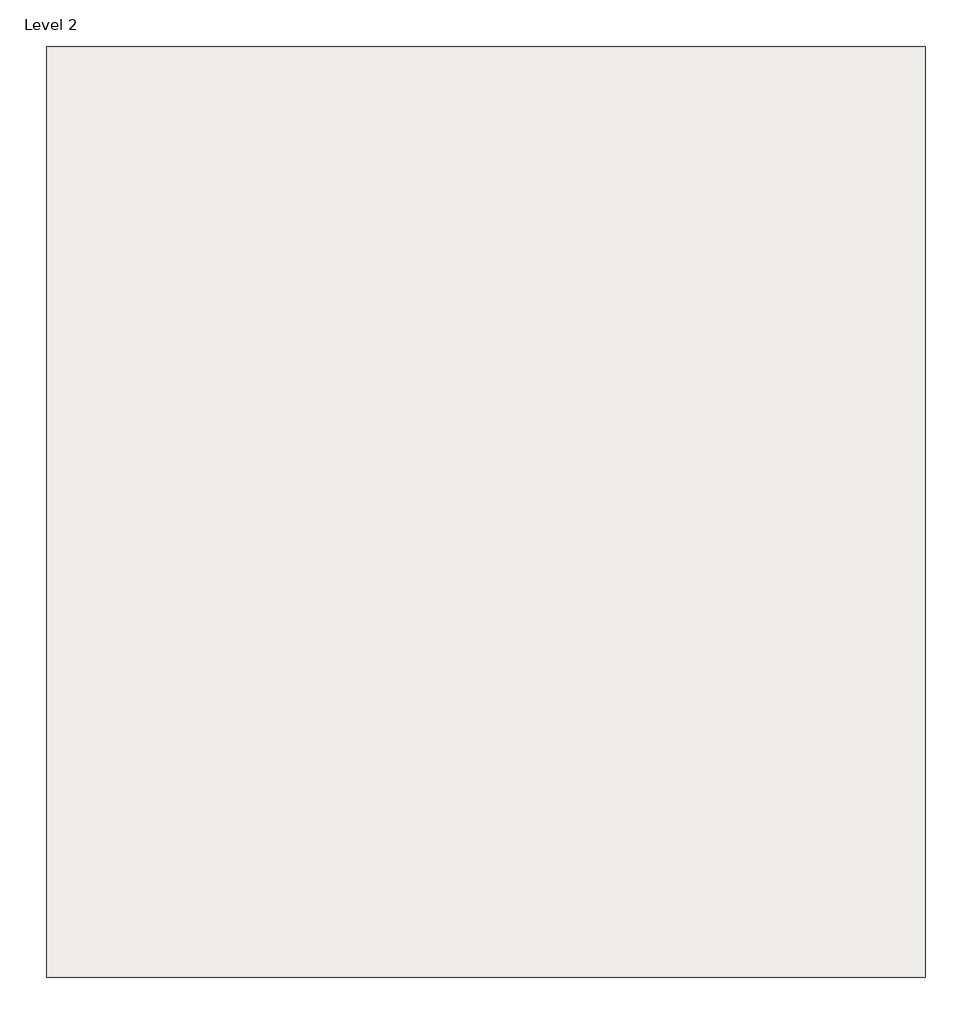
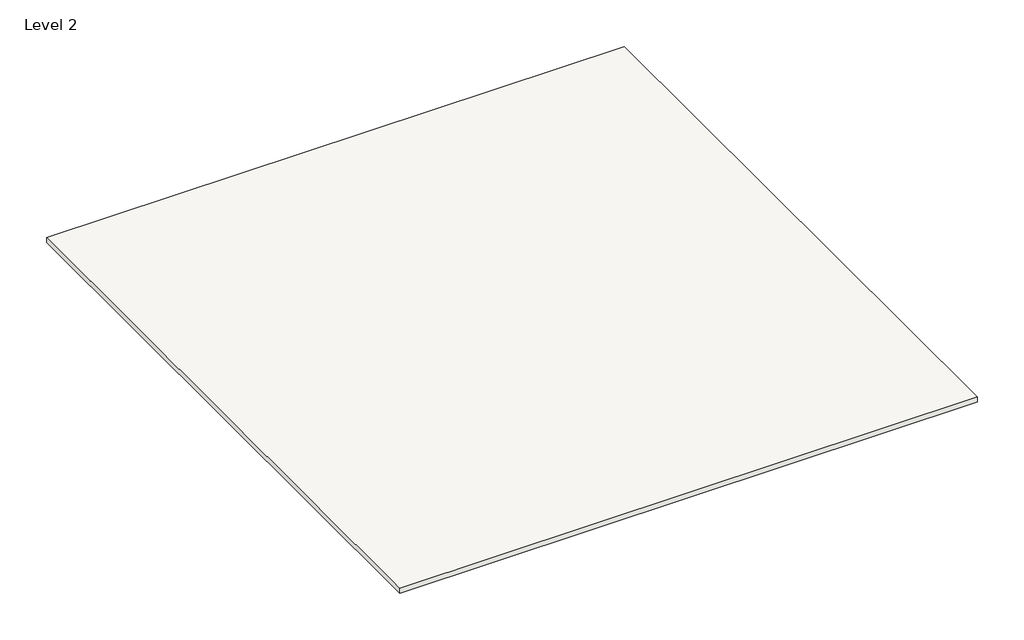
# One storey: 1 slab.
"""IFC4 building model written with IfcOpenShell, lengths in millimetres."""

from ifc_helpers import new_model, si_unit, frame, origin, place, context, project, spatial, polyline, outline, extrude, element, save

model = new_model("IFC4")

# Units and contexts
model_context = context("Model", 3, world=origin())
ifc_project = project(units=[si_unit("LENGTHUNIT", "METRE", prefix="MILLI")], contexts=[model_context])

# Site, building, storey
site = spatial("IfcSite", under=ifc_project)
building = spatial("IfcBuilding", under=site)
storey = spatial("IfcBuildingStorey", under=building, Name="Level 2", Elevation=3657.6)

# Slab
placement = place(None, origin())
element("IfcSlab", 1, ObjectType="6\" floor", at=placement, inside=storey, context=model_context, shape_type="SweptSolid", body=[
    extrude(outline(polyline([(8524.8750735, 9396.8050084), (8524.8750735, -9005.4949916), (-8848.7249265, -9005.4949916), (-8848.7249265, 9396.8050084), (8524.8750735, 9396.8050084)])), frame((0.0, 0.0, 3657.6), z_axis=(0.0, 0.0, 1.0), x_axis=(1.0, 0.0, 0.0)), (0.0, 0.0, 1.0), 152.4),
])

save(model, "model.ifc")

# Revit data of these elements
# Type "6\" floor"
#   Assembly Code = "B1010"
#   Function = 0
#   Layers, outside or top first: 0' - 6" no material (function 1)
# Element 1 (IfcSlab, "6\" floor")
#   Height Offset From Level = 0' - 6"
#   Phase Created = New Construction
#   Materials on its faces: "Default Floor"
# Materials
#   "Default Floor": colour RGB 128 128 128, transparency 0, Cost = 0
